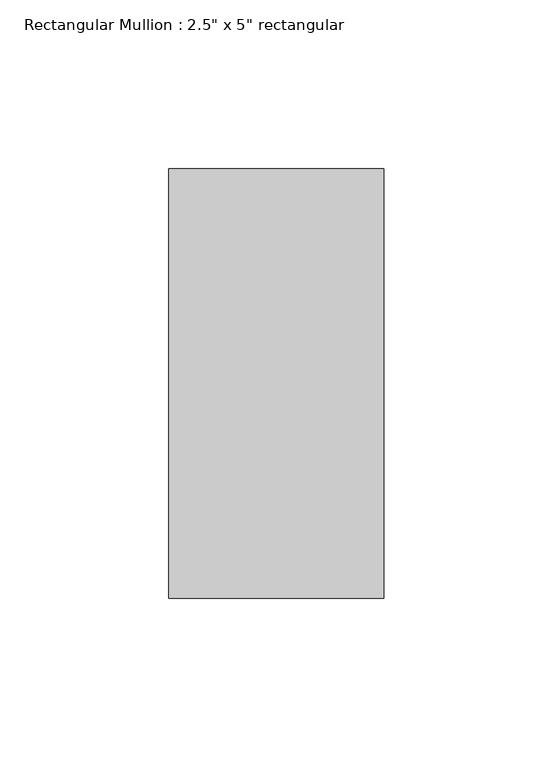
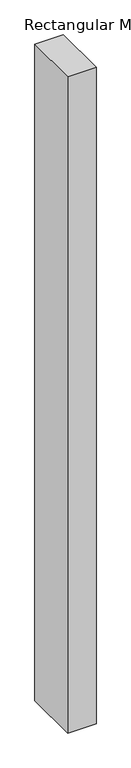
"""IFC4 building model written with IfcOpenShell, lengths in millimetres: member geometry."""

from ifc_helpers import new_model, si_unit, frame, origin, place, context, project, spatial, polyline, outline, extrude, source, transform, mapped, element, save


def member_9389d775(model_context):
    return source(origin(), model_context, "Body", "SweptSolid", [
        extrude(outline(polyline([(0.0, 63.5), (0.0, -63.5), (-63.5, -63.5), (-63.5, 63.5), (0.0, 63.5)])), frame((0.0, 0.0, -1553.4572054), z_axis=(0.0, 0.0, 1.0), x_axis=(1.0, 0.0, 0.0)), (0.0, 0.0, 1.0), 1553.4572054),
    ])


if __name__ == "__main__":
    model = new_model("IFC4")
    model_context = context("Model", 3, world=origin())
    ifc_project = project(units=[si_unit("LENGTHUNIT", "METRE", prefix="MILLI")], contexts=[model_context])
    site = spatial("IfcSite", under=ifc_project)
    building = spatial("IfcBuilding", under=site)
    placement = place(None, origin())
    member_shape = member_9389d775(model_context)
    element("IfcMember", 1, ObjectType="Rectangular Mullion : 2.5\" x 5\" rectangular", at=placement, inside=building, context=model_context, shape_type="MappedRepresentation", body=[
        mapped(member_shape, transform((0.0, 0.0, 0.0), x_axis=(1.0, 0.0, 0.0), y_axis=(0.0, 1.0, 0.0), z_axis=(0.0, 0.0, 1.0))),
    ])
    save(model, "model.ifc")

# Revit data of these elements
# Type "Rectangular Mullion : 2.5\" x 5\" rectangular"
#   built-in parameter 1007304 = 0.416667 (stored number, unit not read)
#   built-in parameter 1007301 = 0.104167 (stored number, unit not read)
#   built-in parameter 1007300 = 0.104167 (stored number, unit not read)
# Element 1 (IfcMember, "Rectangular Mullion : 2.5\" x 5\" rectangular")
#   Materials on its faces: "Aluminum"
# Materials
#   "Aluminum": class "Metal", colour RGB 247 247 247, transparency 0, Description = "Aluminum 6061", Cost = 0
